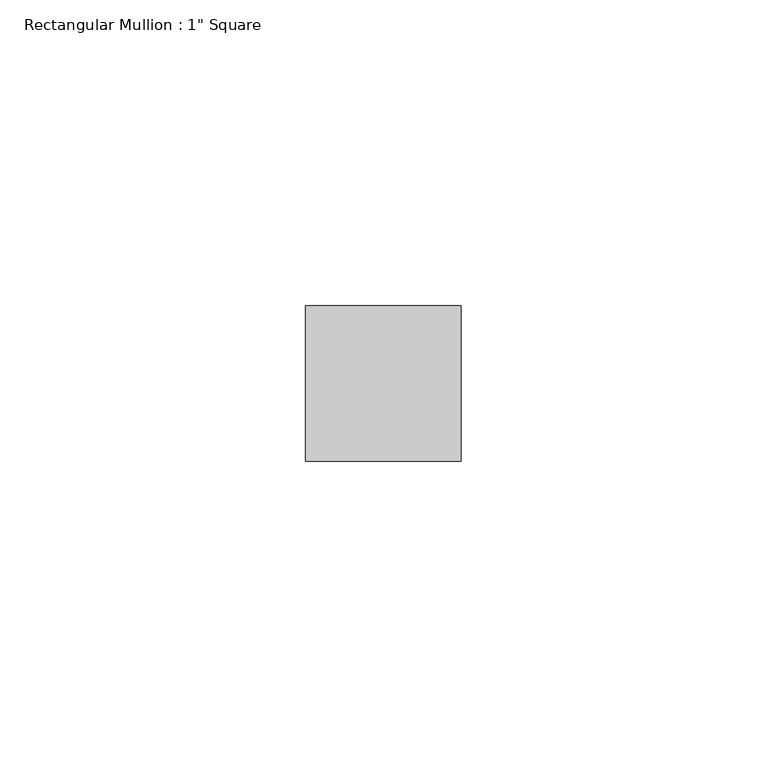
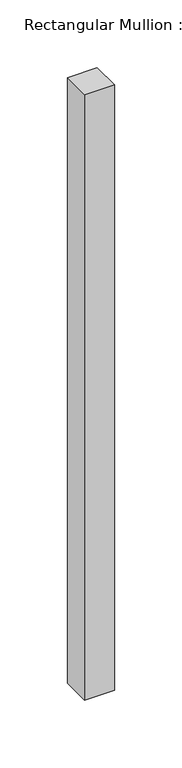
"""IFC4 building model written with IfcOpenShell, lengths in millimetres: member geometry."""

from ifc_helpers import new_model, si_unit, frame, origin, place, context, project, spatial, polyline, outline, extrude, source, transform, mapped, element, save


def member_80fbcd94(model_context):
    return source(origin(), model_context, "Body", "SweptSolid", [
        extrude(outline(polyline([(12.7, 12.7), (12.7, -12.7), (-12.7, -12.7), (-12.7, 12.7), (12.7, 12.7)])), frame((0.0, 0.0, -546.1), z_axis=(0.0, 0.0, 1.0), x_axis=(1.0, 0.0, 0.0)), (0.0, 0.0, 1.0), 546.1),
    ])


if __name__ == "__main__":
    model = new_model("IFC4")
    model_context = context("Model", 3, world=origin())
    ifc_project = project(units=[si_unit("LENGTHUNIT", "METRE", prefix="MILLI")], contexts=[model_context])
    site = spatial("IfcSite", under=ifc_project)
    building = spatial("IfcBuilding", under=site)
    placement = place(None, origin())
    member_shape = member_80fbcd94(model_context)
    element("IfcMember", 1, ObjectType="Rectangular Mullion : 1\" Square", at=placement, inside=building, context=model_context, shape_type="MappedRepresentation", body=[
        mapped(member_shape, transform((0.0, 0.0, 0.0), x_axis=(1.0, 0.0, 0.0), y_axis=(0.0, 1.0, 0.0), z_axis=(0.0, 0.0, 1.0))),
    ])
    save(model, "model.ifc")

# Revit data of these elements
# Type "Rectangular Mullion : 1\" Square"
#   built-in parameter 1007304 = 0.0833333 (stored number, unit not read)
#   built-in parameter 1007301 = 0.0416667 (stored number, unit not read)
#   built-in parameter 1007300 = 0.0416667 (stored number, unit not read)
